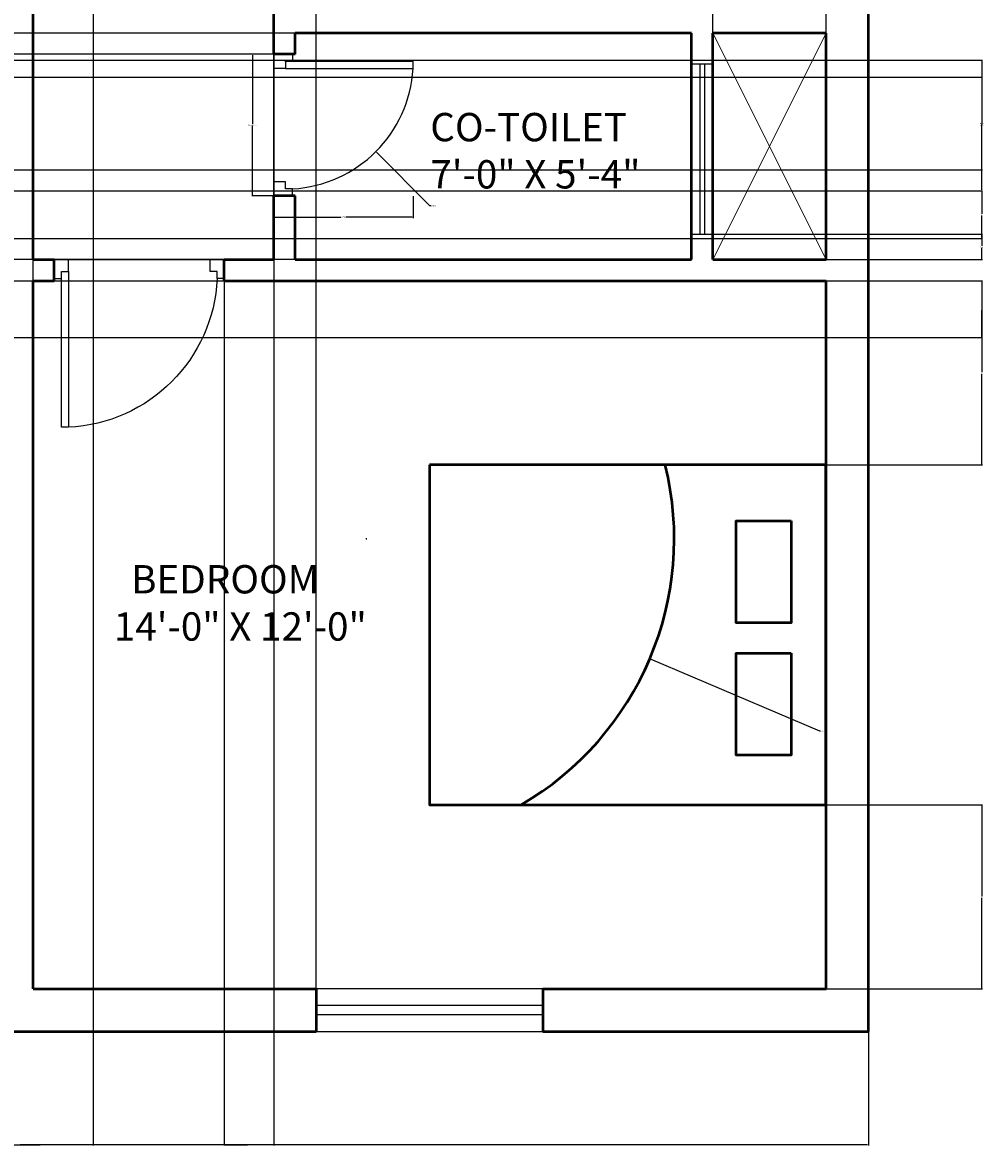
# Model space of a CAD drawing. Units: inches. Extents: x 2330 to 2739, y 947 to 1475.
# Tile 2 of 6: x 2535 to 2739, y 947 to 1185. Entities that reach past the tile are written whole.
import ezdxf

# ---------------------------------------------------------------- set-up
doc = ezdxf.new("R2010")
doc.units = ezdxf.units.IN
for name, color, linetype, lineweight in [('A-ANNO-DIMS', 2, 'Continuous', 18), ('A-AREA-IDEN', 7, 'Continuous', 25), ('door', 150, 'Continuous', 25), ('furniture', 9, 'Continuous', 18), ('railing', 224, 'Continuous', 13), ('wall', 7, 'Continuous', 50), ('window', 40, 'Continuous', 25)]:
    doc.layers.add(name, color=color, linetype=linetype, lineweight=lineweight)
doc.styles.get("Standard").update_dxf_attribs({"font": 'arial.ttf'})
doc.dimstyles.get("Standard").update_dxf_attribs({"dimtxt": 0.18, "dimasz": 0.18, "dimexe": 0.18, "dimexo": 0.0625, "dimgap": 0.09, "dimtad": 0, "dimtih": 1, "dimtoh": 1, "dimdec": 4, "dimzin": 0, "dimdsep": 46, "dimtxsty": 'Standard', "dimcen": 0.09, "dimadec": 0, "dimazin": 0, "dimtfac": 1, "dimtdec": 4, "dimtofl": 0, "dimtmove": 0, "dimatfit": 3, "dimfxl": 1, "dimtolj": 1, "dimtzin": 0, "dimarcsym": 0})

# ---------------------------------------------------------------- blocks, each defined once
blk = doc.blocks.new('d2')
at = {"layer": 'door'}
blk.add_line((2897.27, 1250.29), (2927.27, 1250.29), dxfattribs=at)
blk.add_lwpolyline([(2898.77, 1252.79), (2900.27, 1252.79), (2900.27, 1279.79), (2898.77, 1279.79)], close=True, dxfattribs=at)
for points in [[(2900.27, 1250.29), (2897.27, 1250.29), (2897.27, 1254.29), (2898.77, 1254.29), (2898.77, 1252.79), (2900.27, 1252.79), (2900.27, 1250.29)], [(2924.27, 1250.29), (2927.27, 1250.29), (2927.27, 1254.29), (2925.77, 1254.29), (2925.77, 1252.79), (2924.27, 1252.79), (2924.27, 1250.29)]]:
    blk.add_lwpolyline(points, dxfattribs=at)
blk.add_arc((2898.77, 1252.79), 27.04, 3.1798, 86.8202, dxfattribs=at)
blk = doc.blocks.new('w1')
at = {"layer": 'window'}
for p, q in [((2786.57, 1274.71), (2786.57, 1226.71)), ((2788.57, 1274.71), (2788.57, 1226.71))]:
    blk.add_line(p, q, dxfattribs=at)
blk.add_lwpolyline([(2783.07, 1226.71), (2792.07, 1226.71), (2792.07, 1274.71), (2783.07, 1274.71)], close=True, dxfattribs=at)
blk = doc.blocks.new('w3')
at = {"layer": 'window'}
for p, q in [((2833.35, 1386.77), (2833.35, 1350.77)), ((2834.35, 1386.77), (2834.35, 1350.77))]:
    blk.add_line(p, q, dxfattribs=at)
blk.add_lwpolyline([(2831.6, 1350.77), (2836.1, 1350.77), (2836.1, 1386.77), (2831.6, 1386.77)], close=True, dxfattribs=at)
blk = doc.blocks.new('d1')
at = {"layer": 'door'}
blk.add_line((2897.27, 1313.4), (2933.27, 1313.4), dxfattribs=at)
blk.add_lwpolyline([(2898.77, 1315.9), (2900.27, 1315.9), (2900.27, 1348.9), (2898.77, 1348.9)], close=True, dxfattribs=at)
for points in [[(2900.27, 1313.4), (2897.27, 1313.4), (2897.27, 1317.4), (2898.77, 1317.4), (2898.77, 1315.9), (2900.27, 1315.9), (2900.27, 1313.4)], [(2930.27, 1313.4), (2933.27, 1313.4), (2933.27, 1317.4), (2931.77, 1317.4), (2931.77, 1315.9), (2930.27, 1315.9), (2930.27, 1313.4)]]:
    blk.add_lwpolyline(points, dxfattribs=at)
blk.add_arc((2898.77, 1315.9), 33.03, 2.6026, 87.3974, dxfattribs=at)
blk = doc.blocks.new('BED')
at = {"layer": 'wall'}
for points in [[(2902.88, 1364.87), (2974.88, 1364.87), (2974.88, 1448.87), (2902.88, 1448.87)], [(2914.71, 1441.49), (2936.34, 1441.49), (2936.34, 1429.82), (2914.71, 1429.82)], [(2942.76, 1441.49), (2964.39, 1441.49), (2964.39, 1429.82), (2942.76, 1429.82)]]:
    blk.add_lwpolyline(points, close=True, dxfattribs=at)
blk.add_arc((2918.5, 1351.51), 65.2, 30.1485, 103.8594, dxfattribs=at)
blk = doc.blocks.new('*D14')
at = {"layer": 'A-ANNO-DIMS', "color": 0, "lineweight": -2, "transparency": 16777216}
for p, q in [((2588.62, 1178.28), (2584, 1178.28)), ((2584.18, 1178.1), (2584.18, 1163.47)), ((2584.18, 1148.46), (2584.18, 1163.1)), ((2588.62, 1148.28), (2584, 1148.28))]:
    blk.add_line(p, q, dxfattribs=at)
at = {"layer": 'A-ANNO-DIMS', "color": 0, "transparency": 16777216}
for points in [[(2584.15, 1178.1), (2584.21, 1178.1), (2584.18, 1178.28)], [(2584.15, 1148.46), (2584.21, 1148.46), (2584.18, 1148.28)]]:
    blk.add_solid(points, dxfattribs=at)
at = {"layer": 'Defpoints', "color": 0, "transparency": 16777216}
for p in [(2588.68, 1178.28), (2584.18, 1148.28), (2588.68, 1148.28)]:
    blk.add_point(p, dxfattribs=at)
at = {"layer": 'A-ANNO-DIMS', "color": 0, "transparency": 16777216, "insert": (2584.18, 1163.28), "char_height": 0.18, "attachment_point": 5}
blk.add_mtext('\\A1;DOOR D2 30 TYP.', dxfattribs=at)
blk = doc.blocks.new('*D15')
at = {"layer": 'A-ANNO-DIMS', "color": 0, "lineweight": -2, "transparency": 16777216}
for p, q in [((2588.68, 1148.22), (2588.68, 1143.6)), ((2618.18, 1148.22), (2618.18, 1143.6)), ((2588.86, 1143.78), (2602.9, 1143.78)), ((2618, 1143.78), (2603.96, 1143.78))]:
    blk.add_line(p, q, dxfattribs=at)
at = {"layer": 'A-ANNO-DIMS', "color": 0, "transparency": 16777216}
for points in [[(2588.86, 1143.81), (2588.86, 1143.75), (2588.68, 1143.78)], [(2618, 1143.81), (2618, 1143.75), (2618.18, 1143.78)]]:
    blk.add_solid(points, dxfattribs=at)
at = {"layer": 'Defpoints', "color": 0, "transparency": 16777216}
for p in [(2588.68, 1148.28), (2618.18, 1148.28), (2618.18, 1143.78)]:
    blk.add_point(p, dxfattribs=at)
at = {"layer": 'A-ANNO-DIMS', "color": 0, "transparency": 16777216, "insert": (2603.43, 1143.78), "char_height": 0.18, "attachment_point": 5}
blk.add_mtext('\\A1;30 TYP.', dxfattribs=at)
blk = doc.blocks.new('*D24')
at = {"layer": 'A-ANNO-DIMS', "color": 0, "lineweight": -2, "transparency": 16777216}
for p, q in [((2354.68, 971.22), (2354.68, 947.1)), ((2714.68, 971.22), (2714.68, 947.1)), ((2354.86, 947.28), (2534.39, 947.28)), ((2714.5, 947.28), (2534.97, 947.28))]:
    blk.add_line(p, q, dxfattribs=at)
at = {"layer": 'A-ANNO-DIMS', "color": 0, "transparency": 16777216}
for points in [[(2354.86, 947.31), (2354.86, 947.25), (2354.68, 947.28)], [(2714.5, 947.31), (2714.5, 947.25), (2714.68, 947.28)]]:
    blk.add_solid(points, dxfattribs=at)
at = {"layer": 'Defpoints', "color": 0, "transparency": 16777216}
for p in [(2354.68, 971.28), (2714.68, 971.28), (2714.68, 947.28)]:
    blk.add_point(p, dxfattribs=at)
at = {"layer": 'A-ANNO-DIMS', "color": 0, "transparency": 16777216, "insert": (2534.68, 947.28), "char_height": 0.18, "attachment_point": 5}
blk.add_mtext('\\A1;360', dxfattribs=at)
blk = doc.blocks.new('*D27')
at = {"layer": 'A-ANNO-DIMS', "color": 0, "lineweight": -2, "transparency": 16777216}
for p, q in [((2537.68, 980.34), (2537.68, 1475.46)), ((2537.86, 1475.28), (2567.46, 1475.28)), ((2597.5, 1475.28), (2567.9, 1475.28)), ((2597.68, 980.34), (2597.68, 1475.46))]:
    blk.add_line(p, q, dxfattribs=at)
at = {"layer": 'A-ANNO-DIMS', "color": 0, "transparency": 16777216}
for points in [[(2537.86, 1475.31), (2537.86, 1475.25), (2537.68, 1475.28)], [(2597.5, 1475.31), (2597.5, 1475.25), (2597.68, 1475.28)]]:
    blk.add_solid(points, dxfattribs=at)
at = {"layer": 'Defpoints', "color": 0, "transparency": 16777216}
for p in [(2597.68, 1475.28), (2537.68, 980.28), (2597.68, 980.28)]:
    blk.add_point(p, dxfattribs=at)
at = {"layer": 'A-ANNO-DIMS', "color": 0, "transparency": 16777216, "insert": (2567.68, 1475.28), "char_height": 0.18, "attachment_point": 5}
blk.add_mtext('\\A1;60', dxfattribs=at)
blk = doc.blocks.new('*D28')
at = {"layer": 'A-ANNO-DIMS', "color": 0, "lineweight": -2, "transparency": 16777216}
for p, q in [((2705.74, 1019.28), (2738.86, 1019.28)), ((2738.68, 1019.1), (2738.68, 999.96)), ((2738.68, 980.46), (2738.68, 999.6)), ((2705.74, 980.28), (2738.86, 980.28))]:
    blk.add_line(p, q, dxfattribs=at)
at = {"layer": 'A-ANNO-DIMS', "color": 0, "transparency": 16777216}
for points in [[(2738.65, 1019.1), (2738.71, 1019.1), (2738.68, 1019.28)], [(2738.65, 980.46), (2738.71, 980.46), (2738.68, 980.28)]]:
    blk.add_solid(points, dxfattribs=at)
at = {"layer": 'Defpoints', "color": 0, "transparency": 16777216}
for p in [(2705.68, 1019.28), (2738.68, 1019.28), (2705.68, 980.28)]:
    blk.add_point(p, dxfattribs=at)
at = {"layer": 'A-ANNO-DIMS', "color": 0, "transparency": 16777216, "insert": (2738.68, 999.78), "char_height": 0.18, "attachment_point": 5}
blk.add_mtext('\\A1;39', dxfattribs=at)
blk = doc.blocks.new('*D30')
at = {"layer": 'A-ANNO-DIMS', "color": 0, "lineweight": -2, "transparency": 16777216}
for p, q in [((2677.12, 1182.78), (2330.5, 1182.78)), ((2330.68, 1182.6), (2330.68, 1158.96)), ((2330.68, 1134.96), (2330.68, 1158.6)), ((2677.12, 1134.78), (2330.5, 1134.78))]:
    blk.add_line(p, q, dxfattribs=at)
at = {"layer": 'A-ANNO-DIMS', "color": 0, "transparency": 16777216}
for points in [[(2330.65, 1182.6), (2330.71, 1182.6), (2330.68, 1182.78)], [(2330.65, 1134.96), (2330.71, 1134.96), (2330.68, 1134.78)]]:
    blk.add_solid(points, dxfattribs=at)
at = {"layer": 'Defpoints', "color": 0, "transparency": 16777216}
for p in [(2330.68, 1182.78), (2677.18, 1182.78), (2677.18, 1134.78)]:
    blk.add_point(p, dxfattribs=at)
at = {"layer": 'A-ANNO-DIMS', "color": 0, "transparency": 16777216, "insert": (2330.68, 1158.78), "char_height": 0.18, "attachment_point": 5}
blk.add_mtext('\\A1;48', dxfattribs=at)
blk = doc.blocks.new('*D36')
at = {"layer": 'A-ANNO-DIMS', "color": 0, "lineweight": -2, "transparency": 16777216}
for p, q in [((2528.68, 1394.22), (2528.68, 947.1)), ((2550.43, 1394.22), (2550.43, 947.1)), ((2528.86, 947.28), (2539.16, 947.28)), ((2550.25, 947.28), (2539.95, 947.28))]:
    blk.add_line(p, q, dxfattribs=at)
at = {"layer": 'A-ANNO-DIMS', "color": 0, "transparency": 16777216}
for points in [[(2528.86, 947.31), (2528.86, 947.25), (2528.68, 947.28)], [(2550.25, 947.31), (2550.25, 947.25), (2550.43, 947.28)]]:
    blk.add_solid(points, dxfattribs=at)
at = {"layer": 'Defpoints', "color": 0, "transparency": 16777216}
for p in [(2528.68, 1394.28), (2550.43, 1394.28), (2550.43, 947.28)]:
    blk.add_point(p, dxfattribs=at)
at = {"layer": 'A-ANNO-DIMS', "color": 0, "transparency": 16777216, "insert": (2539.55, 947.28), "char_height": 0.18, "attachment_point": 5}
blk.add_mtext('\\A1;21.75', dxfattribs=at)
blk = doc.blocks.new('*D38')
at = {"layer": 'A-ANNO-DIMS', "color": 0, "lineweight": -2, "transparency": 16777216}
for p, q in [((2537.68, 1134.84), (2537.68, 1475.46)), ((2537.86, 1475.28), (2562.98, 1475.28)), ((2588.5, 1475.28), (2563.38, 1475.28)), ((2588.68, 1134.84), (2588.68, 1475.46))]:
    blk.add_line(p, q, dxfattribs=at)
at = {"layer": 'A-ANNO-DIMS', "color": 0, "transparency": 16777216}
for points in [[(2537.86, 1475.31), (2537.86, 1475.25), (2537.68, 1475.28)], [(2588.5, 1475.31), (2588.5, 1475.25), (2588.68, 1475.28)]]:
    blk.add_solid(points, dxfattribs=at)
at = {"layer": 'Defpoints', "color": 0, "transparency": 16777216}
for p in [(2588.68, 1475.28), (2537.68, 1134.78), (2588.68, 1134.78)]:
    blk.add_point(p, dxfattribs=at)
at = {"layer": 'A-ANNO-DIMS', "color": 0, "transparency": 16777216, "insert": (2563.18, 1475.28), "char_height": 0.18, "attachment_point": 5}
blk.add_mtext('\\A1;51', dxfattribs=at)
blk = doc.blocks.new('*D39')
at = {"layer": 'A-ANNO-DIMS', "color": 0, "lineweight": -2, "transparency": 16777216}
for p, q in [((2578.18, 1134.72), (2578.18, 947.1)), ((2588.68, 1134.72), (2588.68, 947.1)), ((2578.36, 947.28), (2583.11, 947.28)), ((2588.5, 947.28), (2583.74, 947.28))]:
    blk.add_line(p, q, dxfattribs=at)
at = {"layer": 'A-ANNO-DIMS', "color": 0, "transparency": 16777216}
for points in [[(2578.36, 947.31), (2578.36, 947.25), (2578.18, 947.28)], [(2588.5, 947.31), (2588.5, 947.25), (2588.68, 947.28)]]:
    blk.add_solid(points, dxfattribs=at)
at = {"layer": 'Defpoints', "color": 0, "transparency": 16777216}
for p in [(2578.18, 1134.78), (2588.68, 1134.78), (2588.68, 947.28)]:
    blk.add_point(p, dxfattribs=at)
at = {"layer": 'A-ANNO-DIMS', "color": 0, "transparency": 16777216, "insert": (2583.43, 947.28), "char_height": 0.18, "attachment_point": 5}
blk.add_mtext('\\A1;10.5', dxfattribs=at)
blk = doc.blocks.new('*D42')
at = {"layer": 'A-ANNO-DIMS', "color": 0, "lineweight": -2, "transparency": 16777216}
for p, q in [((2681.74, 1140.21), (2738.86, 1140.21)), ((2738.68, 1140.03), (2738.68, 1137.68)), ((2738.68, 1134.96), (2738.68, 1137.31)), ((2681.74, 1134.78), (2738.86, 1134.78))]:
    blk.add_line(p, q, dxfattribs=at)
at = {"layer": 'A-ANNO-DIMS', "color": 0, "transparency": 16777216}
for points in [[(2738.65, 1140.03), (2738.71, 1140.03), (2738.68, 1140.21)], [(2738.65, 1134.96), (2738.71, 1134.96), (2738.68, 1134.78)]]:
    blk.add_solid(points, dxfattribs=at)
at = {"layer": 'Defpoints', "color": 0, "transparency": 16777216}
for p in [(2681.68, 1140.21), (2681.68, 1134.78), (2738.68, 1134.78)]:
    blk.add_point(p, dxfattribs=at)
at = {"layer": 'A-ANNO-DIMS', "color": 0, "transparency": 16777216, "insert": (2738.68, 1137.5), "char_height": 0.18, "attachment_point": 5}
blk.add_mtext('\\A1;5.426', dxfattribs=at)
blk = doc.blocks.new('*D43')
at = {"layer": 'A-ANNO-DIMS', "color": 0, "lineweight": -2, "transparency": 16777216}
for p, q in [((2593.12, 1182.78), (2330.5, 1182.78)), ((2330.68, 1182.6), (2330.68, 1180.71)), ((2330.68, 1178.46), (2330.68, 1180.35)), ((2593.12, 1178.28), (2330.5, 1178.28))]:
    blk.add_line(p, q, dxfattribs=at)
at = {"layer": 'A-ANNO-DIMS', "color": 0, "transparency": 16777216}
for points in [[(2330.65, 1182.6), (2330.71, 1182.6), (2330.68, 1182.78)], [(2330.65, 1178.46), (2330.71, 1178.46), (2330.68, 1178.28)]]:
    blk.add_solid(points, dxfattribs=at)
at = {"layer": 'Defpoints', "color": 0, "transparency": 16777216}
for p in [(2593.18, 1182.78), (2330.68, 1178.28), (2593.18, 1178.28)]:
    blk.add_point(p, dxfattribs=at)
at = {"layer": 'A-ANNO-DIMS', "color": 0, "transparency": 16777216, "insert": (2330.68, 1180.53), "char_height": 0.18, "attachment_point": 5}
blk.add_mtext('\\A1;4.5', dxfattribs=at)
blk = doc.blocks.new('*D49')
at = {"layer": 'A-ANNO-DIMS', "color": 0, "lineweight": -2, "transparency": 16777216}
for p, q in [((2475.16, 1177.05), (2738.86, 1177.05)), ((2738.68, 1176.87), (2738.68, 1163.39)), ((2738.68, 1149.54), (2738.68, 1163.02)), ((2475.16, 1149.36), (2738.86, 1149.36))]:
    blk.add_line(p, q, dxfattribs=at)
at = {"layer": 'A-ANNO-DIMS', "color": 0, "transparency": 16777216}
for points in [[(2738.65, 1176.87), (2738.71, 1176.87), (2738.68, 1177.05)], [(2738.65, 1149.54), (2738.71, 1149.54), (2738.68, 1149.36)]]:
    blk.add_solid(points, dxfattribs=at)
at = {"layer": 'Defpoints', "color": 0, "transparency": 16777216}
for p in [(2475.1, 1177.05), (2475.1, 1149.36), (2738.68, 1149.36)]:
    blk.add_point(p, dxfattribs=at)
at = {"layer": 'A-ANNO-DIMS', "color": 0, "transparency": 16777216, "insert": (2738.68, 1163.21), "char_height": 0.18, "attachment_point": 5}
blk.add_mtext('\\A1;27.687', dxfattribs=at)
blk = doc.blocks.new('*D51')
at = {"layer": 'A-ANNO-DIMS', "color": 0, "lineweight": -2, "transparency": 16777216}
for p, q in [((2388.29, 1173.45), (2738.86, 1173.45)), ((2738.68, 1173.27), (2738.68, 1163.81)), ((2738.68, 1153.98), (2738.68, 1163.44)), ((2388.29, 1153.8), (2738.86, 1153.8))]:
    blk.add_line(p, q, dxfattribs=at)
at = {"layer": 'A-ANNO-DIMS', "color": 0, "transparency": 16777216}
for points in [[(2738.65, 1173.27), (2738.71, 1173.27), (2738.68, 1173.45)], [(2738.65, 1153.98), (2738.71, 1153.98), (2738.68, 1153.8)]]:
    blk.add_solid(points, dxfattribs=at)
at = {"layer": 'Defpoints', "color": 0, "transparency": 16777216}
for p in [(2388.23, 1173.45), (2388.23, 1153.8), (2738.68, 1153.8)]:
    blk.add_point(p, dxfattribs=at)
at = {"layer": 'A-ANNO-DIMS', "color": 0, "transparency": 16777216, "insert": (2738.68, 1163.63), "char_height": 0.18, "attachment_point": 5}
blk.add_mtext('\\A1;19.643', dxfattribs=at)
blk = doc.blocks.new('*D55')
at = {"layer": 'A-ANNO-DIMS', "color": 0, "lineweight": -2, "transparency": 16777216}
for p, q in [((2397.62, 1149.36), (2738.86, 1149.36)), ((2738.68, 1149.18), (2738.68, 1144.5)), ((2738.68, 1139.46), (2738.68, 1144.14)), ((2401.99, 1139.28), (2738.86, 1139.28))]:
    blk.add_line(p, q, dxfattribs=at)
at = {"layer": 'A-ANNO-DIMS', "color": 0, "transparency": 16777216}
for points in [[(2738.65, 1149.18), (2738.71, 1149.18), (2738.68, 1149.36)], [(2738.65, 1139.46), (2738.71, 1139.46), (2738.68, 1139.28)]]:
    blk.add_solid(points, dxfattribs=at)
at = {"layer": 'Defpoints', "color": 0, "transparency": 16777216}
for p in [(2397.55, 1149.36), (2738.68, 1149.36), (2401.93, 1139.28)]:
    blk.add_point(p, dxfattribs=at)
at = {"layer": 'A-ANNO-DIMS', "color": 0, "transparency": 16777216, "insert": (2738.68, 1144.32), "char_height": 0.18, "attachment_point": 5}
blk.add_mtext('\\A1;10.08', dxfattribs=at)
blk = doc.blocks.new('*D77')
at = {"layer": 'A-ANNO-DIMS', "color": 0, "lineweight": -2, "transparency": 16777216}
for p, q in [((2705.74, 1130.28), (2738.86, 1130.28)), ((2738.68, 1130.1), (2738.68, 1110.96)), ((2738.68, 1091.46), (2738.68, 1110.6)), ((2705.74, 1091.28), (2738.86, 1091.28))]:
    blk.add_line(p, q, dxfattribs=at)
at = {"layer": 'A-ANNO-DIMS', "color": 0, "transparency": 16777216}
for points in [[(2738.65, 1130.1), (2738.71, 1130.1), (2738.68, 1130.28)], [(2738.65, 1091.46), (2738.71, 1091.46), (2738.68, 1091.28)]]:
    blk.add_solid(points, dxfattribs=at)
at = {"layer": 'Defpoints', "color": 0, "transparency": 16777216}
for p in [(2705.68, 1130.28), (2705.68, 1091.28), (2738.68, 1091.28)]:
    blk.add_point(p, dxfattribs=at)
at = {"layer": 'A-ANNO-DIMS', "color": 0, "transparency": 16777216, "insert": (2738.68, 1110.78), "char_height": 0.18, "attachment_point": 5}
blk.add_mtext('\\A1;39', dxfattribs=at)
blk = doc.blocks.new('*D78')
at = {"layer": 'A-ANNO-DIMS', "color": 0, "lineweight": -2, "transparency": 16777216}
for p, q in [((2681.68, 1182.84), (2681.68, 1475.46)), ((2681.86, 1475.28), (2693.46, 1475.28)), ((2705.5, 1475.28), (2693.9, 1475.28)), ((2705.68, 1182.84), (2705.68, 1475.46))]:
    blk.add_line(p, q, dxfattribs=at)
at = {"layer": 'A-ANNO-DIMS', "color": 0, "transparency": 16777216}
for points in [[(2681.86, 1475.31), (2681.86, 1475.25), (2681.68, 1475.28)], [(2705.5, 1475.31), (2705.5, 1475.25), (2705.68, 1475.28)]]:
    blk.add_solid(points, dxfattribs=at)
at = {"layer": 'Defpoints', "color": 0, "transparency": 16777216}
for p in [(2705.68, 1475.28), (2681.68, 1182.78), (2705.68, 1182.78)]:
    blk.add_point(p, dxfattribs=at)
at = {"layer": 'A-ANNO-DIMS', "color": 0, "transparency": 16777216, "insert": (2693.68, 1475.28), "char_height": 0.18, "attachment_point": 5}
blk.add_mtext('\\A1;24', dxfattribs=at)
blk = doc.blocks.new('*D81')
at = {"layer": 'A-ANNO-DIMS', "color": 0, "lineweight": -2, "transparency": 16777216}
for p, q in [((2480.87, 1130.28), (2738.86, 1130.28)), ((2738.68, 1130.1), (2738.68, 1124.46)), ((2738.68, 1118.46), (2738.68, 1124.1)), ((2480.87, 1118.28), (2738.86, 1118.28))]:
    blk.add_line(p, q, dxfattribs=at)
at = {"layer": 'A-ANNO-DIMS', "color": 0, "transparency": 16777216}
for points in [[(2738.65, 1130.1), (2738.71, 1130.1), (2738.68, 1130.28)], [(2738.65, 1118.46), (2738.71, 1118.46), (2738.68, 1118.28)]]:
    blk.add_solid(points, dxfattribs=at)
at = {"layer": 'Defpoints', "color": 0, "transparency": 16777216}
for p in [(2480.81, 1130.28), (2738.68, 1130.28), (2480.81, 1118.28)]:
    blk.add_point(p, dxfattribs=at)
at = {"layer": 'A-ANNO-DIMS', "color": 0, "transparency": 16777216, "insert": (2738.68, 1124.28), "char_height": 0.18, "attachment_point": 5}
blk.add_mtext('\\A1;12', dxfattribs=at)
blk = doc.blocks.new('*D82')
at = {"layer": 'A-ANNO-DIMS', "color": 0, "lineweight": -2, "transparency": 16777216}
for p, q in [((2608.22, 1075.66), (2608.4, 1075.66)), ((2608.31, 1075.57), (2608.31, 1075.75)), ((2704.35, 1034.91), (2668.5, 1050.12)), ((2704.53, 1034.91), (2704.35, 1034.91))]:
    blk.add_line(p, q, dxfattribs=at)
at = {"layer": 'A-ANNO-DIMS', "color": 0, "transparency": 16777216}
blk.add_solid([(2668.51, 1050.15), (2668.49, 1050.09), (2668.33, 1050.19)], dxfattribs=at)
at = {"layer": 'Defpoints', "color": 0, "transparency": 16777216}
for p in [(2608.31, 1075.66), (2668.33, 1050.19)]:
    blk.add_point(p, dxfattribs=at)
at = {"layer": 'A-ANNO-DIMS', "color": 0, "transparency": 16777216, "insert": (2705.13, 1034.91), "char_height": 0.18, "attachment_point": 5}
blk.add_mtext('\\A1;2X R65.2', dxfattribs=at)
blk = doc.blocks.new('*D83')
at = {"layer": 'A-ANNO-DIMS', "color": 0, "lineweight": -2, "transparency": 16777216}
for p, q in [((2591.09, 1176.78), (2591.27, 1176.78)), ((2591.18, 1176.69), (2591.18, 1176.87)), ((2621.77, 1146.19), (2610.43, 1157.53)), ((2621.95, 1146.19), (2621.77, 1146.19))]:
    blk.add_line(p, q, dxfattribs=at)
at = {"layer": 'A-ANNO-DIMS', "color": 0, "transparency": 16777216}
blk.add_solid([(2610.45, 1157.55), (2610.41, 1157.51), (2610.3, 1157.66)], dxfattribs=at)
at = {"layer": 'Defpoints', "color": 0, "transparency": 16777216}
for p in [(2591.18, 1176.78), (2610.3, 1157.66)]:
    blk.add_point(p, dxfattribs=at)
at = {"layer": 'A-ANNO-DIMS', "color": 0, "transparency": 16777216, "insert": (2622.62, 1146.19), "char_height": 0.18, "attachment_point": 5}
blk.add_mtext('\\A1;3X R27.04', dxfattribs=at)

msp = doc.modelspace()

# ---------------------------------------------------------------- linework, layer by layer
at = {"layer": 'railing'}
for p, q in [((2705.6781, 1182.7823), (2681.6781, 1134.7823)), ((2681.6781, 1182.7823), (2705.6781, 1134.7823))]:
    msp.add_line(p, q, dxfattribs=at)
at = {"layer": 'wall'}
for p, q in [((2714.6781, 971.2823), (2714.6781, 1451.2823)), ((2537.6781, 1134.7823), (2537.6781, 1187.2823)), ((2588.6781, 1178.2823), (2588.6781, 1187.2823)), ((2677.1781, 1182.7823), (2593.1781, 1182.7823)), ((2593.1781, 1178.2823), (2593.1781, 1182.7823)), ((2677.1781, 1134.7823), (2677.1781, 1182.7823)), ((2705.6781, 1182.7823), (2681.6781, 1182.7823)), ((2681.6781, 1134.7823), (2681.6781, 1182.7823)), ((2705.6781, 1134.7823), (2705.6781, 1182.7823)), ((2593.1781, 1178.2823), (2588.6781, 1178.2823)), ((2588.6781, 1134.7823), (2588.6781, 1148.2823)), ((2593.1781, 1148.2823), (2588.6781, 1148.2823)), ((2593.1781, 1134.7823), (2593.1781, 1148.2823)), ((2537.6781, 1134.7823), (2542.1781, 1134.7823)), ((2542.1781, 1130.2823), (2542.1781, 1134.7823)), ((2578.1781, 1130.2823), (2578.1781, 1134.7823)), ((2578.1781, 1134.7823), (2588.6781, 1134.7823)), ((2593.1781, 1134.7823), (2677.1781, 1134.7823)), ((2681.6781, 1134.7823), (2705.6781, 1134.7823)), ((2537.6781, 980.2823), (2537.6781, 1130.2823)), ((2537.6781, 1130.2823), (2542.1781, 1130.2823)), ((2578.1781, 1130.2823), (2705.6781, 1130.2823)), ((2705.6781, 980.2823), (2705.6781, 1130.2823)), ((2537.6781, 980.2823), (2597.6781, 980.2823)), ((2597.6781, 980.2823), (2597.6781, 971.2823)), ((2645.6781, 980.2823), (2645.6781, 971.2823)), ((2645.6781, 980.2823), (2705.6781, 980.2823)), ((2354.6781, 971.2823), (2597.6781, 971.2823)), ((2645.6781, 971.2823), (2714.6781, 971.2823))]:
    msp.add_line(p, q, dxfattribs=at)

# ---------------------------------------------------------------- block references
at = {"layer": 'door', "rotation": 270}
msp.add_blockref('d2', (1338.3871, 4075.5513), dxfattribs=at)
at = {"layer": 'door', "xscale": -1, "rotation": 180}
msp.add_blockref('d1', (-355.0909, 2448.1812), dxfattribs=at)
at = {"layer": 'furniture', "rotation": 270}
msp.add_blockref('BED', (1256.8054, 3994.1666), dxfattribs=at)
at = {"layer": 'window'}
msp.add_blockref('w3', (-154.4186, -210.5664), dxfattribs=at)
at = {"layer": 'window', "rotation": 270}
msp.add_blockref('w1', (1370.9695, 3763.3542), dxfattribs=at)

# ---------------------------------------------------------------- texts
at = {"layer": 'A-AREA-IDEN', "char_height": 6, "attachment_point": 1}
for s, insert in [('CO-TOILET\\P7\'-0" X 5\'-4"', (2621.8392, 1165.8618)), ('  BEDROOM\\P14\'-0" X 12\'-0"', (2554.7838, 1070.0696))]:
    msp.add_mtext_dynamic_manual_height_columns(s, width=63.218259, gutter_width=12.5, heights=[0], dxfattribs=dict(at, insert=insert))

# ---------------------------------------------------------------- dimensions: what is measured, and where the dimension line sits
at = {"layer": 'A-ANNO-DIMS'}
for base, p1, p2, override, picture, middle in [((2597.6781, 1475.2843), (2537.6781, 980.2823), (2597.6781, 980.2823), {"dimdec": 0, "dimlfac": 1, "dimrnd": 0, "dimzin": 0, "dimdsep": 46, "dimlunit": 2}, '*D27', (2567.6781, 1475.2843)), ((2588.6781, 1475.2843), (2537.6781, 1134.7823), (2588.6781, 1134.7823), {"dimdec": 0, "dimlfac": 1, "dimrnd": 0, "dimzin": 0, "dimdsep": 46, "dimlunit": 2}, '*D38', (2563.1781, 1475.2843)), ((2705.6781, 1475.2843), (2681.6781, 1182.7823), (2705.6781, 1182.7823), {"dimdec": 0, "dimlfac": 1, "dimrnd": 0, "dimzin": 0, "dimdsep": 46, "dimlunit": 2}, '*D78', (2693.6781, 1475.2843)), ((2550.4281, 947.2803), (2528.6781, 1394.2823), (2550.4281, 1394.2823), {"dimdec": 2, "dimlfac": 1, "dimrnd": 0, "dimzin": 0, "dimdsep": 46, "dimlunit": 2}, '*D36', (2539.5531, 947.2803)), ((2588.6781, 947.2803), (2578.1781, 1134.7823), (2588.6781, 1134.7823), {"dimdec": 1, "dimlfac": 1, "dimrnd": 0, "dimzin": 0, "dimdsep": 46, "dimlunit": 2}, '*D39', (2583.4281, 947.2803)), ((2714.6781, 947.2803), (2354.6781, 971.2823), (2714.6781, 971.2823), {"dimdec": 0, "dimlfac": 1, "dimrnd": 0, "dimzin": 0, "dimdsep": 46, "dimlunit": 2}, '*D24', (2534.6781, 947.2803))]:
    dim = msp.add_linear_dim(base=base, p1=p1, p2=p2, dimstyle='Standard', override=override, dxfattribs=at)
    dim.commit()
    dim.dimension.update_dxf_attribs({"geometry": picture, "text_midpoint": middle})
for base, p1, p2, override, picture, middle in [((2330.6761, 1182.7823), (2677.1781, 1134.7823), (2677.1781, 1182.7823), {"dimdec": 0, "dimlfac": 1, "dimrnd": 0, "dimzin": 0, "dimdsep": 46, "dimlunit": 2}, '*D30', (2330.6761, 1158.7823)), ((2330.6761, 1178.2823), (2593.1781, 1182.7823), (2593.1781, 1178.2823), {"dimdec": 1, "dimlfac": 1, "dimrnd": 0, "dimzin": 0, "dimdsep": 46, "dimlunit": 2}, '*D43', (2330.6761, 1180.5323)), ((2738.6801, 1149.3617), (2475.0968, 1177.0487), (2475.0968, 1149.3617), {"dimdec": 3, "dimlfac": 1, "dimrnd": 0, "dimzin": 0, "dimdsep": 46, "dimlunit": 2}, '*D49', (2738.6801, 1163.2052)), ((2738.6801, 1153.8045), (2388.2258, 1173.4475), (2388.2258, 1153.8045), {"dimdec": 3, "dimlfac": 1, "dimrnd": 0, "dimzin": 0, "dimdsep": 46, "dimlunit": 2}, '*D51', (2738.6801, 1163.626)), ((2738.6801, 1149.3617), (2401.9281, 1139.2823), (2397.5542, 1149.3617), {"dimdec": 2, "dimlfac": 1, "dimrnd": 0, "dimzin": 0, "dimdsep": 46, "dimlunit": 2}, '*D55', (2738.6801, 1144.322)), ((2738.68012, 1134.78225), (2681.67812, 1140.20782), (2681.67812, 1134.78225), {"dimdec": 3, "dimlfac": 1, "dimrnd": 0, "dimzin": 0, "dimdsep": 46, "dimlunit": 2}, '*D42', (2738.68012, 1137.49504)), ((2738.6801, 1130.2823), (2480.806, 1118.2823), (2480.806, 1130.2823), {"dimdec": 0, "dimlfac": 1, "dimrnd": 0, "dimzin": 0, "dimdsep": 46, "dimlunit": 2}, '*D81', (2738.6801, 1124.2823)), ((2738.6801, 1091.2823), (2705.6781, 1130.2823), (2705.6781, 1091.2823), {"dimdec": 0, "dimlfac": 1, "dimrnd": 0, "dimzin": 0, "dimdsep": 46, "dimlunit": 2}, '*D77', (2738.6801, 1110.7823)), ((2738.6801, 1019.2823), (2705.6781, 980.2823), (2705.6781, 1019.2823), {"dimdec": 0, "dimlfac": 1, "dimrnd": 0, "dimzin": 0, "dimdsep": 46, "dimlunit": 2}, '*D28', (2738.6801, 999.7823))]:
    dim = msp.add_linear_dim(base=base, p1=p1, p2=p2, angle=90, dimstyle='Standard', override=override, dxfattribs=at)
    dim.commit()
    dim.dimension.update_dxf_attribs({"geometry": picture, "text_midpoint": middle})
dim = msp.add_linear_dim(base=(2584.1781, 1148.2823), p1=(2588.6781, 1178.2823), p2=(2588.6781, 1148.2823), angle=270, text='DOOR D2 <> TYP.', dimstyle='Standard', override={"dimdec": 0, "dimlfac": 1, "dimrnd": 0, "dimzin": 0, "dimdsep": 46, "dimlunit": 2}, dxfattribs=at)
dim.commit()
dim.dimension.update_dxf_attribs({"geometry": '*D14', "text_midpoint": (2584.1781, 1163.2823)})
for center, mpoint, text, override, picture, middle in [((2591.1781, 1176.7823), (2610.2993, 1157.6607), '3X <>', {"dimdec": 2, "dimlfac": 1, "dimrnd": 0, "dimzin": 0, "dimdsep": 46, "dimlunit": 2}, '*D83', (2622.6247, 1146.1878)), ((2608.3126, 1075.6638), (2668.3329, 1050.192), '2X <>', {"dimdec": 1, "dimlfac": 1, "dimrnd": 0, "dimzin": 0, "dimdsep": 46, "dimlunit": 2}, '*D82', (2705.129, 1034.909))]:
    dim = msp.add_radius_dim(center=center, mpoint=mpoint, text=text, dimstyle='Standard', override=override, dxfattribs=at)
    dim.commit()
    dim.dimension.update_dxf_attribs({"geometry": picture, "text_midpoint": middle, "dimtype": 164})
dim = msp.add_linear_dim(base=(2618.1781181692, 1143.7822535815), p1=(2588.6781181692, 1148.2822535815), p2=(2618.1781181692, 1148.2822535815), text='<> TYP.', dimstyle='Standard', override={"dimdec": 0, "dimlfac": 1, "dimrnd": 0, "dimzin": 0, "dimdsep": 46, "dimlunit": 2}, dxfattribs=at)
dim.commit()
dim.dimension.update_dxf_attribs({"geometry": '*D15', "text_midpoint": (2603.4281181692, 1143.7822535815)})

doc.saveas('drawing.dxf')
